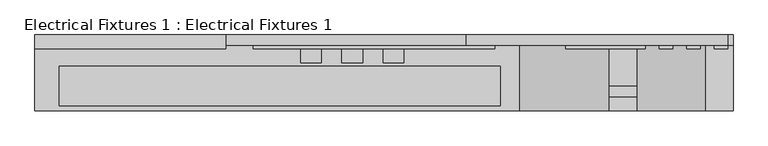
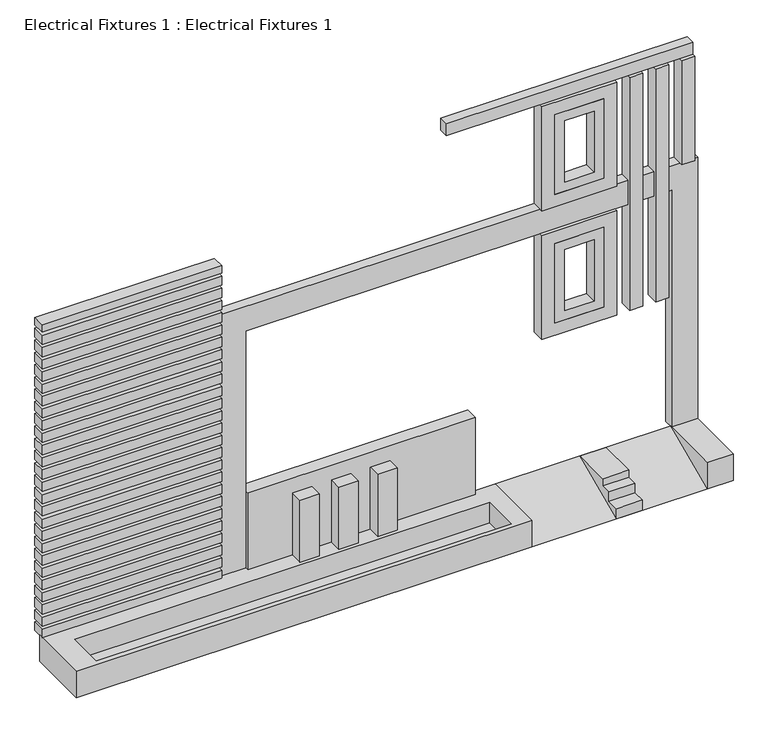
"""IFC4 building model written with IfcOpenShell, lengths in millimetres: proxy geometry, Electrical Fixtures 1 : Electrical Fixtures 1."""

from ifc_helpers import new_model, si_unit, frame, origin, origin_with_axes, place, context, project, spatial, polyline, outline, extrude, faceted_brep, source, transform, mapped, element, save


def electrical_fixtures_1_electrical_fixtures_1_7c594ec0(model_context):
    return source(origin(), model_context, "Body", "SolidModel", [
        faceted_brep([(3260.6353535, -16726.7330955, 660.4), (3260.6353535, -16726.7330955, 0.0), (3260.6353535, -15240.8330955, 0.0), (3260.6353535, -15240.8330955, 660.4), (-7454.7186876, -16726.7330955, 660.4), (-7454.7186876, -15240.8330955, 660.4), (-7454.7186876, -15240.8330955, 0.0), (-7454.7186876, -16726.7330955, 0.0), (-6918.9587128, -16619.1790654, 660.4), (-6918.9587128, -15738.2380402, 660.4), (2834.6412872, -15738.2380402, 660.4), (2834.6412872, -16619.1790654, 660.4), (-6918.9587128, -16619.1790654, 144.4887841), (2834.6412872, -16619.1790654, 144.4887841), (2834.6412872, -15738.2380402, 144.4887841), (-6918.9587128, -15738.2380402, 144.4887841)], [[[0, 1, 2, 3]], [[4, 5, 6, 7]], [[2, 1, 7, 6]], [[3, 2, 6, 5]], [[0, 3, 5, 4], [8, 9, 10, 11]], [[1, 0, 4, 7]], [[12, 13, 14, 15]], [[12, 15, 9, 8]], [[15, 14, 10, 9]], [[14, 13, 11, 10]], [[13, 12, 8, 11]]]),
        extrude(outline(polyline([(-16167.9330955, 660.4), (-15240.8330955, 660.4), (-15240.8330955, 0.0), (-16726.7330955, 0.0), (-16726.7330955, 254.0), (-16421.9330955, 254.0), (-16421.9330955, 482.6), (-16167.9330955, 482.6), (-16167.9330955, 660.4)])), frame((5245.2813124, 0.0, 0.0), z_axis=(1.0, 0.0, 0.0), x_axis=(0.0, 1.0, 0.0)), (0.0, 0.0, 1.0), 609.6),
        extrude(outline(polyline([(7988.4813124, -15240.8330955), (7988.4813124, -16726.7330955), (7378.8813124, -16726.7330955), (7378.8813124, -15240.8330955), (7988.4813124, -15240.8330955)])), origin_with_axes(), (0.0, 0.0, 1.0), 660.4),
        extrude(outline(polyline([(-16726.7330955, 0.0), (-15240.8330955, 660.4), (-15240.8330955, 0.0), (-16726.7330955, 0.0)])), frame((3260.6353535, 0.0, 0.0), z_axis=(1.0, 0.0, 0.0), x_axis=(0.0, 1.0, 0.0)), (0.0, 0.0, 1.0), 4118.2459589),
        extrude(outline(polyline([(7467.6, 4590.6893946), (7467.6, 5740.985334), (9448.8, 5740.985334), (9448.8, 4590.6893946), (7467.6, 4590.6893946)]), holes=[polyline([(7696.2, 4819.2893946), (9220.2, 4819.2893946), (9220.2, 5512.385334), (7696.2, 5512.385334), (7696.2, 4819.2893946)])]), frame((0.0, -15355.1330955, 0.0), z_axis=(0.0, 1.0, 0.0), x_axis=(0.0, 0.0, 1.0)), (0.0, 0.0, 1.0), 304.8),
        extrude(outline(polyline([(6248.4, 4590.6893946), (4267.2, 4590.6893946), (4267.2, 5740.985334), (6248.4, 5740.985334), (6248.4, 4590.6893946)]), holes=[polyline([(6019.8, 4819.2893946), (6019.8, 5512.385334), (4495.8, 5512.385334), (4495.8, 4819.2893946), (6019.8, 4819.2893946)])]), frame((0.0, -15355.1330955, 0.0), z_axis=(0.0, 1.0, 0.0), x_axis=(0.0, 0.0, 1.0)), (0.0, 0.0, 1.0), 304.8),
        extrude(outline(polyline([(-1120.882453, -15659.9330955), (-1578.082453, -15659.9330955), (-1578.082453, -15050.3330955), (-1120.882453, -15050.3330955), (-1120.882453, -15659.9330955)])), frame((0.0, 0.0, 660.4), z_axis=(0.0, 0.0, 1.0), x_axis=(1.0, 0.0, 0.0)), (0.0, 0.0, 1.0), 1543.6755822),
        extrude(outline(polyline([(-206.482453, -15659.9330955), (-663.682453, -15659.9330955), (-663.682453, -15050.3330955), (-206.482453, -15050.3330955), (-206.482453, -15659.9330955)])), frame((0.0, 0.0, 660.4), z_axis=(0.0, 0.0, 1.0), x_axis=(1.0, 0.0, 0.0)), (0.0, 0.0, 1.0), 1543.6755822),
        extrude(outline(polyline([(707.917547, -15659.9330955), (250.717547, -15659.9330955), (250.717547, -15050.3330955), (707.917547, -15050.3330955), (707.917547, -15659.9330955)])), frame((0.0, 0.0, 660.4), z_axis=(0.0, 0.0, 1.0), x_axis=(1.0, 0.0, 0.0)), (0.0, 0.0, 1.0), 1543.6755822),
        extrude(outline(polyline([(7264.985334, -15355.1330955), (6960.185334, -15355.1330955), (6960.185334, -15050.3330955), (7264.985334, -15050.3330955), (7264.985334, -15355.1330955)])), frame((0.0, 0.0, 3962.4), z_axis=(0.0, 0.0, 1.0), x_axis=(1.0, 0.0, 0.0)), (0.0, 0.0, 1.0), 5791.2),
        extrude(outline(polyline([(6655.385334, -15355.1330955), (6350.585334, -15355.1330955), (6350.585334, -15050.3330955), (6655.385334, -15050.3330955), (6655.385334, -15355.1330955)])), frame((0.0, 0.0, 3962.4), z_axis=(0.0, 0.0, 1.0), x_axis=(1.0, 0.0, 0.0)), (0.0, 0.0, 1.0), 5791.2),
        extrude(outline(polyline([(3962.4, 6045.785334), (6553.2, 6045.785334), (6553.2, 4285.8893946), (3962.4, 4285.8893946), (3962.4, 6045.785334)]), holes=[polyline([(6248.4, 5740.985334), (4267.2, 5740.985334), (4267.2, 4590.6893946), (6248.4, 4590.6893946), (6248.4, 5740.985334)])]), frame((0.0, -15355.1330955, 0.0), z_axis=(0.0, 1.0, 0.0), x_axis=(0.0, 0.0, 1.0)), (0.0, 0.0, 1.0), 304.8),
        extrude(outline(polyline([(7874.585334, -15355.1330955), (7569.785334, -15355.1330955), (7569.785334, -15050.3330955), (7874.585334, -15050.3330955), (7874.585334, -15355.1330955)])), frame((0.0, 0.0, 7162.8), z_axis=(0.0, 0.0, 1.0), x_axis=(1.0, 0.0, 0.0)), (0.0, 0.0, 1.0), 2590.8),
        extrude(outline(polyline([(9753.6, 6045.785334), (9753.6, 4285.8893946), (7162.8, 4285.8893946), (7162.8, 6045.785334), (9753.6, 6045.785334)]), holes=[polyline([(7467.6, 5740.985334), (7467.6, 4590.6893946), (9448.8, 4590.6893946), (9448.8, 5740.985334), (7467.6, 5740.985334)])]), frame((0.0, -15355.1330955, 0.0), z_axis=(0.0, 1.0, 0.0), x_axis=(0.0, 0.0, 1.0)), (0.0, 0.0, 1.0), 304.8),
        extrude(outline(polyline([(2721.2721831, -15355.1330955), (-2628.7186876, -15355.1330955), (-2628.7186876, -15050.3330955), (2721.2721831, -15050.3330955), (2721.2721831, -15355.1330955)])), frame((0.0, 0.0, 660.4), z_axis=(0.0, 0.0, 1.0), x_axis=(1.0, 0.0, 0.0)), (0.0, 0.0, 1.0), 1913.6),
        extrude(outline(polyline([(-3238.3186876, -15355.1330955), (-7454.7186876, -15355.1330955), (-7454.7186876, -15050.3330955), (-3238.3186876, -15050.3330955), (-3238.3186876, -15355.1330955)])), frame((0.0, 0.0, 8255.9295469), z_axis=(0.0, 0.0, 1.0), x_axis=(1.0, 0.0, 0.0)), (0.0, 0.0, 1.0), 176.8704531),
        extrude(outline(polyline([(-3238.3186876, -15355.1330955), (-7454.7186876, -15355.1330955), (-7454.7186876, -15050.3330955), (-3238.3186876, -15050.3330955), (-3238.3186876, -15355.1330955)])), frame((0.0, 0.0, 660.4), z_axis=(0.0, 0.0, 1.0), x_axis=(1.0, 0.0, 0.0)), (0.0, 0.0, 1.0), 204.1295469),
        extrude(outline(polyline([(-3238.3186876, -15355.1330955), (-7454.7186876, -15355.1330955), (-7454.7186876, -15050.3330955), (-3238.3186876, -15050.3330955), (-3238.3186876, -15355.1330955)])), frame((0.0, 0.0, 7951.1295469), z_axis=(0.0, 0.0, 1.0), x_axis=(1.0, 0.0, 0.0)), (0.0, 0.0, 1.0), 228.6),
        extrude(outline(polyline([(-3238.3186876, -15355.1330955), (-7454.7186876, -15355.1330955), (-7454.7186876, -15050.3330955), (-3238.3186876, -15050.3330955), (-3238.3186876, -15355.1330955)])), frame((0.0, 0.0, 7646.3295469), z_axis=(0.0, 0.0, 1.0), x_axis=(1.0, 0.0, 0.0)), (0.0, 0.0, 1.0), 228.6),
        extrude(outline(polyline([(-3238.3186876, -15355.1330955), (-7454.7186876, -15355.1330955), (-7454.7186876, -15050.3330955), (-3238.3186876, -15050.3330955), (-3238.3186876, -15355.1330955)])), frame((0.0, 0.0, 7341.5295469), z_axis=(0.0, 0.0, 1.0), x_axis=(1.0, 0.0, 0.0)), (0.0, 0.0, 1.0), 228.6),
        extrude(outline(polyline([(-3238.3186876, -15355.1330955), (-7454.7186876, -15355.1330955), (-7454.7186876, -15050.3330955), (-3238.3186876, -15050.3330955), (-3238.3186876, -15355.1330955)])), frame((0.0, 0.0, 7036.7295469), z_axis=(0.0, 0.0, 1.0), x_axis=(1.0, 0.0, 0.0)), (0.0, 0.0, 1.0), 228.6),
        extrude(outline(polyline([(-3238.3186876, -15355.1330955), (-7454.7186876, -15355.1330955), (-7454.7186876, -15050.3330955), (-3238.3186876, -15050.3330955), (-3238.3186876, -15355.1330955)])), frame((0.0, 0.0, 6731.9295469), z_axis=(0.0, 0.0, 1.0), x_axis=(1.0, 0.0, 0.0)), (0.0, 0.0, 1.0), 228.6),
        extrude(outline(polyline([(-3238.3186876, -15355.1330955), (-7454.7186876, -15355.1330955), (-7454.7186876, -15050.3330955), (-3238.3186876, -15050.3330955), (-3238.3186876, -15355.1330955)])), frame((0.0, 0.0, 6427.1295469), z_axis=(0.0, 0.0, 1.0), x_axis=(1.0, 0.0, 0.0)), (0.0, 0.0, 1.0), 228.6),
        extrude(outline(polyline([(-3238.3186876, -15355.1330955), (-7454.7186876, -15355.1330955), (-7454.7186876, -15050.3330955), (-3238.3186876, -15050.3330955), (-3238.3186876, -15355.1330955)])), frame((0.0, 0.0, 6122.3295469), z_axis=(0.0, 0.0, 1.0), x_axis=(1.0, 0.0, 0.0)), (0.0, 0.0, 1.0), 228.6),
        extrude(outline(polyline([(-3238.3186876, -15355.1330955), (-7454.7186876, -15355.1330955), (-7454.7186876, -15050.3330955), (-3238.3186876, -15050.3330955), (-3238.3186876, -15355.1330955)])), frame((0.0, 0.0, 5817.5295469), z_axis=(0.0, 0.0, 1.0), x_axis=(1.0, 0.0, 0.0)), (0.0, 0.0, 1.0), 228.6),
        extrude(outline(polyline([(-3238.3186876, -15355.1330955), (-7454.7186876, -15355.1330955), (-7454.7186876, -15050.3330955), (-3238.3186876, -15050.3330955), (-3238.3186876, -15355.1330955)])), frame((0.0, 0.0, 5512.7295469), z_axis=(0.0, 0.0, 1.0), x_axis=(1.0, 0.0, 0.0)), (0.0, 0.0, 1.0), 228.6),
        extrude(outline(polyline([(-3238.3186876, -15355.1330955), (-7454.7186876, -15355.1330955), (-7454.7186876, -15050.3330955), (-3238.3186876, -15050.3330955), (-3238.3186876, -15355.1330955)])), frame((0.0, 0.0, 5207.9295469), z_axis=(0.0, 0.0, 1.0), x_axis=(1.0, 0.0, 0.0)), (0.0, 0.0, 1.0), 228.6),
        extrude(outline(polyline([(-3238.3186876, -15355.1330955), (-7454.7186876, -15355.1330955), (-7454.7186876, -15050.3330955), (-3238.3186876, -15050.3330955), (-3238.3186876, -15355.1330955)])), frame((0.0, 0.0, 4903.1295469), z_axis=(0.0, 0.0, 1.0), x_axis=(1.0, 0.0, 0.0)), (0.0, 0.0, 1.0), 228.6),
        extrude(outline(polyline([(-3238.3186876, -15355.1330955), (-7454.7186876, -15355.1330955), (-7454.7186876, -15050.3330955), (-3238.3186876, -15050.3330955), (-3238.3186876, -15355.1330955)])), frame((0.0, 0.0, 4598.3295469), z_axis=(0.0, 0.0, 1.0), x_axis=(1.0, 0.0, 0.0)), (0.0, 0.0, 1.0), 228.6),
        extrude(outline(polyline([(-3238.3186876, -15355.1330955), (-7454.7186876, -15355.1330955), (-7454.7186876, -15050.3330955), (-3238.3186876, -15050.3330955), (-3238.3186876, -15355.1330955)])), frame((0.0, 0.0, 4293.5295469), z_axis=(0.0, 0.0, 1.0), x_axis=(1.0, 0.0, 0.0)), (0.0, 0.0, 1.0), 228.6),
        extrude(outline(polyline([(-3238.3186876, -15355.1330955), (-7454.7186876, -15355.1330955), (-7454.7186876, -15050.3330955), (-3238.3186876, -15050.3330955), (-3238.3186876, -15355.1330955)])), frame((0.0, 0.0, 3988.7295469), z_axis=(0.0, 0.0, 1.0), x_axis=(1.0, 0.0, 0.0)), (0.0, 0.0, 1.0), 228.6),
        extrude(outline(polyline([(-3238.3186876, -15355.1330955), (-7454.7186876, -15355.1330955), (-7454.7186876, -15050.3330955), (-3238.3186876, -15050.3330955), (-3238.3186876, -15355.1330955)])), frame((0.0, 0.0, 3683.9295469), z_axis=(0.0, 0.0, 1.0), x_axis=(1.0, 0.0, 0.0)), (0.0, 0.0, 1.0), 228.6),
        extrude(outline(polyline([(-3238.3186876, -15355.1330955), (-7454.7186876, -15355.1330955), (-7454.7186876, -15050.3330955), (-3238.3186876, -15050.3330955), (-3238.3186876, -15355.1330955)])), frame((0.0, 0.0, 3379.1295469), z_axis=(0.0, 0.0, 1.0), x_axis=(1.0, 0.0, 0.0)), (0.0, 0.0, 1.0), 228.6),
        extrude(outline(polyline([(-3238.3186876, -15355.1330955), (-7454.7186876, -15355.1330955), (-7454.7186876, -15050.3330955), (-3238.3186876, -15050.3330955), (-3238.3186876, -15355.1330955)])), frame((0.0, 0.0, 3074.3295469), z_axis=(0.0, 0.0, 1.0), x_axis=(1.0, 0.0, 0.0)), (0.0, 0.0, 1.0), 228.6),
        extrude(outline(polyline([(-3238.3186876, -15355.1330955), (-7454.7186876, -15355.1330955), (-7454.7186876, -15050.3330955), (-3238.3186876, -15050.3330955), (-3238.3186876, -15355.1330955)])), frame((0.0, 0.0, 2769.5295469), z_axis=(0.0, 0.0, 1.0), x_axis=(1.0, 0.0, 0.0)), (0.0, 0.0, 1.0), 228.6),
        extrude(outline(polyline([(-3238.3186876, -15355.1330955), (-7454.7186876, -15355.1330955), (-7454.7186876, -15050.3330955), (-3238.3186876, -15050.3330955), (-3238.3186876, -15355.1330955)])), frame((0.0, 0.0, 2464.7295469), z_axis=(0.0, 0.0, 1.0), x_axis=(1.0, 0.0, 0.0)), (0.0, 0.0, 1.0), 228.6),
        extrude(outline(polyline([(-3238.3186876, -15355.1330955), (-7454.7186876, -15355.1330955), (-7454.7186876, -15050.3330955), (-3238.3186876, -15050.3330955), (-3238.3186876, -15355.1330955)])), frame((0.0, 0.0, 2159.9295469), z_axis=(0.0, 0.0, 1.0), x_axis=(1.0, 0.0, 0.0)), (0.0, 0.0, 1.0), 228.6),
        extrude(outline(polyline([(-3238.3186876, -15355.1330955), (-7454.7186876, -15355.1330955), (-7454.7186876, -15050.3330955), (-3238.3186876, -15050.3330955), (-3238.3186876, -15355.1330955)])), frame((0.0, 0.0, 1855.1295469), z_axis=(0.0, 0.0, 1.0), x_axis=(1.0, 0.0, 0.0)), (0.0, 0.0, 1.0), 228.6),
        extrude(outline(polyline([(-3238.3186876, -15355.1330955), (-7454.7186876, -15355.1330955), (-7454.7186876, -15050.3330955), (-3238.3186876, -15050.3330955), (-3238.3186876, -15355.1330955)])), frame((0.0, 0.0, 1550.3295469), z_axis=(0.0, 0.0, 1.0), x_axis=(1.0, 0.0, 0.0)), (0.0, 0.0, 1.0), 228.6),
        extrude(outline(polyline([(-3238.3186876, -15355.1330955), (-7454.7186876, -15355.1330955), (-7454.7186876, -15050.3330955), (-3238.3186876, -15050.3330955), (-3238.3186876, -15355.1330955)])), frame((0.0, 0.0, 1245.5295469), z_axis=(0.0, 0.0, 1.0), x_axis=(1.0, 0.0, 0.0)), (0.0, 0.0, 1.0), 228.6),
        extrude(outline(polyline([(-3238.3186876, -15355.1330955), (-7454.7186876, -15355.1330955), (-7454.7186876, -15050.3330955), (-3238.3186876, -15050.3330955), (-3238.3186876, -15355.1330955)])), frame((0.0, 0.0, 940.7295469), z_axis=(0.0, 0.0, 1.0), x_axis=(1.0, 0.0, 0.0)), (0.0, 0.0, 1.0), 228.6),
        extrude(outline(polyline([(7162.8, -3238.3186876), (660.4, -3238.3186876), (660.4, -2628.7186876), (6553.2, -2628.7186876), (6553.2, 7378.8813124), (660.4, 7378.8813124), (660.4, 7988.4813124), (7162.8, 7988.4813124), (7162.8, -3238.3186876)])), frame((0.0, -15278.9330955, 0.0), z_axis=(0.0, 1.0, 0.0), x_axis=(0.0, 0.0, 1.0)), (0.0, 0.0, 1.0), 228.6),
        extrude(outline(polyline([(7874.585334, -15278.9330955), (2083.385334, -15278.9330955), (2083.385334, -15050.3330955), (7874.585334, -15050.3330955), (7874.585334, -15278.9330955)])), frame((0.0, 0.0, 9754.6364288), z_axis=(0.0, 0.0, 1.0), x_axis=(1.0, 0.0, 0.0)), (0.0, 0.0, 1.0), 304.8),
    ])


if __name__ == "__main__":
    model = new_model("IFC4")
    model_context = context("Model", 3, world=origin())
    ifc_project = project(units=[si_unit("LENGTHUNIT", "METRE", prefix="MILLI")], contexts=[model_context])
    site = spatial("IfcSite", under=ifc_project)
    building = spatial("IfcBuilding", under=site)
    placement = place(None, origin())
    electrical_fixtures_1_electrical_fixtures_1_shape = electrical_fixtures_1_electrical_fixtures_1_7c594ec0(model_context)
    element("IfcBuildingElementProxy", 1, Name="Electrical Fixtures 1 : Electrical Fixtures 1", ObjectType="Electrical Fixtures 1 : Electrical Fixtures 1", at=placement, inside=building, context=model_context, shape_type="MappedRepresentation", body=[
        mapped(electrical_fixtures_1_electrical_fixtures_1_shape, transform((0.0, 0.0, 0.0), x_axis=(1.0, 0.0, 0.0), y_axis=(0.0, 1.0, 0.0), z_axis=(0.0, 0.0, 1.0))),
    ])
    save(model, "model.ifc")

# Revit data of these elements
# Element 1 (IfcBuildingElementProxy, "Electrical Fixtures 1 : Electrical Fixtures 1")
#   Materials on its faces: "brown", "Concrete, Precast", "black"
# Materials
#   "brown": class "Generic", colour RGB 89 45 45, transparency 0, Cost = 0
#   "Concrete, Precast": class "Concrete", colour RGB 198 187 187, transparency 0, Description = "Precast concrete", Cost = 0
#   "black": class "Generic", colour RGB 92 92 92, transparency 0, Cost = 0
